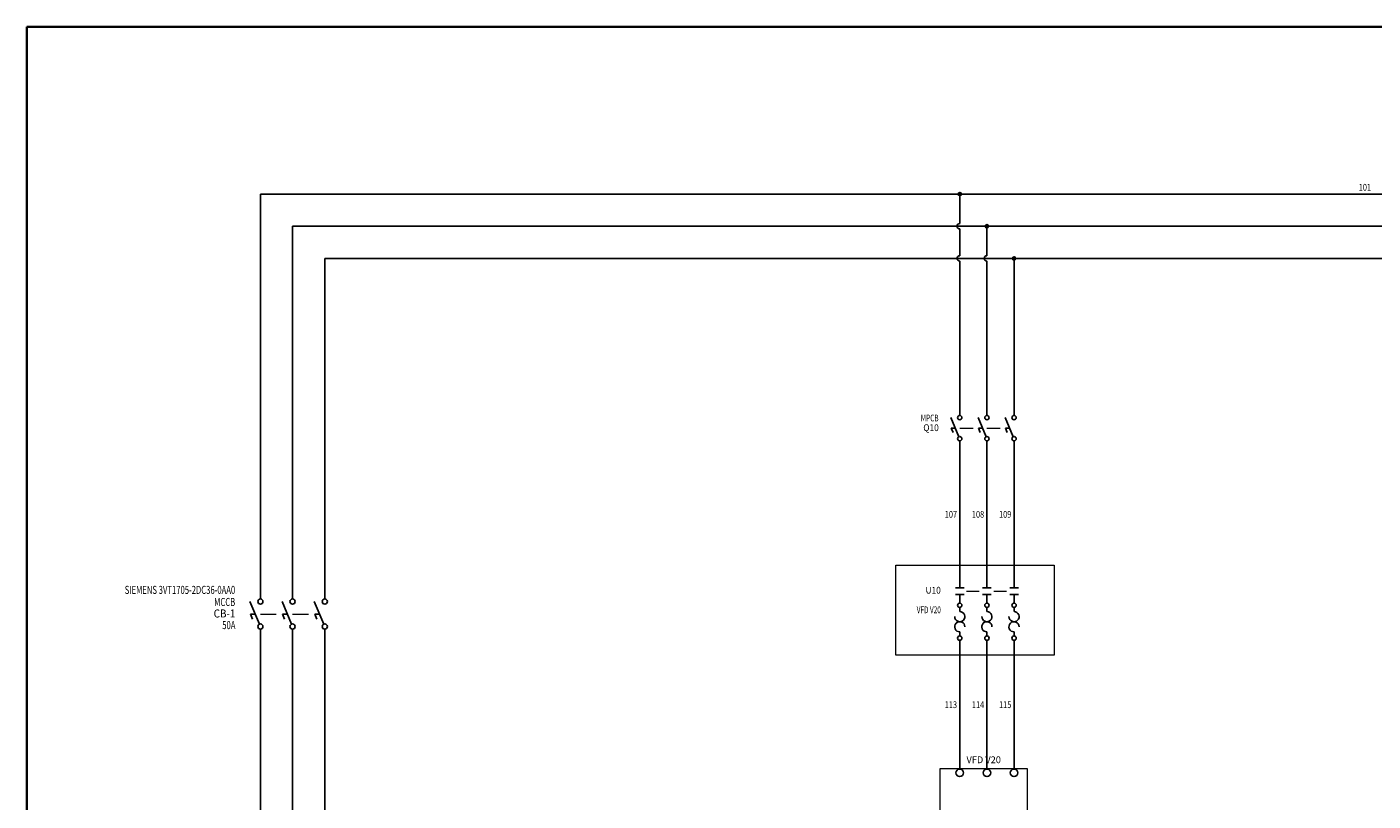
# Model space of a CAD drawing. Units: inches. Extents: x 12.5 to 62, y 4.7 to 37.4.
# Tile 3 of 5: x 12.5 to 37.3, y 23.1 to 37.4. Entities that reach past the tile are written whole.
import ezdxf
from ezdxf.enums import TextEntityAlignment as Align

# ---------------------------------------------------------------- set-up
doc = ezdxf.new("R2010")
doc.units = ezdxf.units.IN
doc.header["$MEASUREMENT"] = 0
for name, color, linetype, lineweight in [('16AWG-BLU', 182, 'Continuous', 25), ('16AWG-GRNYEL', 60, 'Continuous', 25), ('16AWG-RED', 1, 'Continuous', 25), ('E-ANNO-TEXT', 92, 'Continuous', 18), ('E-ANNO-TTLB', 7, 'Continuous', 35), ('LINK', 9, 'Continuous', 13), ('LOCBOX', 7, 'Continuous', 18), ('SYMS', 7, 'Continuous', 25), ('WIRENO', 72, 'Continuous', 18)]:
    doc.layers.add(name, color=color, linetype=linetype, lineweight=lineweight)
for name, color, linetype in [('DESCCHILD', 20, 'Continuous'), ('LOC', 8, 'Continuous'), ('MISC', 7, 'Continuous'), ('TAGS', 150, 'Continuous')]:
    doc.layers.add(name, color=color, linetype=linetype)
doc.styles.get("Standard").update_dxf_attribs({"font": 'arial.ttf'})
doc.styles.add('WD', font='romans.shx')

# ---------------------------------------------------------------- blocks, each defined once
blk = doc.blocks.new('VDS11')
for p, q in [((-0.016, -0.157), (-0.163, 0.195)), ((-0.081, 0), (-0.156, 0)), ((-0.124, -0.078), (-0.156, 0))]:
    blk.add_line(p, q)
for centre in [(0, 0.194), (0, -0.194)]:
    blk.add_circle(centre, 0.0403)
at = {"style": 'WD'}
for tag, width, p in [('INST', 0.7, (-0.391, 0.312)), ('LOC', 0.7, (-0.391, 0.125)), ('TAG1', 0.9, (-0.388, -0.054)), ('RATING1', 0.7, (-0.388, -0.234)), ('DESC1', 0.7, (-0.387, -0.422)), ('DESC2', 0.7, (-0.388, -0.609))]:
    blk.add_attdef(tag, text='', height=0.125, dxfattribs=dict(at, width=width)).set_placement(p, align=Align.RIGHT)
for tag, height, flags, p in [('TERM01', 0.125, 8, (-0.069, 0.258)), ('CONTACT', 0.0125, 9, (-0.083, -0.067)), ('FAMILY', 0.0125, 9, (-0.1, -0.046)), ('MFG', 0.0125, 9, (-0.1, -0.11)), ('CAT', 0.0125, 9, (-0.1, -0.091))]:
    blk.add_attdef(tag, text='', height=height, dxfattribs=dict(at, flags=flags)).set_placement(p, align=Align.RIGHT)
at = {"style": 'WD', "flags": 1}
for tag, p in [('X2TERM01', (0, 0.234)), ('X8TERM02', (0, -0.234))]:
    blk.add_attdef(tag, p, '', height=0.0125, dxfattribs=at)
at = {"style": 'WD'}
for tag, p in [('X4LINK', (-0.254, 0)), ('X1LINK', (0, 0))]:
    blk.add_attdef(tag, p, '', height=0.0125, dxfattribs=at)
at = {"style": 'WD', "width": 0.7}
blk.add_attdef('XREF', (0.161, -0.047), '', height=0.125, dxfattribs=at)
at = {"style": 'WD', "flags": 9}
blk.add_attdef('ASSYCODE', text='', height=0.0125, dxfattribs=at).set_placement((-0.115, -0.137), align=Align.CENTER)
at = {"style": 'WD', "flags": 8}
blk.add_attdef('TERM02', text='', height=0.125, dxfattribs=at).set_placement((-0.051, -0.267), align=Align.TOP_RIGHT)
blk = doc.blocks.new('VDS21')
for p, q in [((-0.016, -0.157), (-0.163, 0.195)), ((-0.081, 0), (-0.156, 0)), ((-0.124, -0.078), (-0.156, 0))]:
    blk.add_line(p, q)
for centre in [(0, 0.194), (0, -0.194)]:
    blk.add_circle(centre, 0.0403)
at = {"style": 'WD'}
for tag, width, p in [('INST', 0.7, (-0.373, 0.406)), ('LOC', 0.7, (-0.373, 0.221)), ('TAG2', 0.9, (-0.373, 0.031)), ('XREF', 0.7, (-0.37, -0.155)), ('DESC1', 0.7, (-0.37, -0.344)), ('DESC2', 0.7, (-0.37, -0.531))]:
    blk.add_attdef(tag, text='', height=0.125, dxfattribs=dict(at, width=width)).set_placement(p, align=Align.RIGHT)
for tag, height, flags, p in [('TERM01', 0.125, 8, (-0.069, 0.258)), ('CONTACT', 0.0125, 9, (-0.083, -0.106)), ('FAMILY', 0.0125, 9, (-0.1, -0.046))]:
    blk.add_attdef(tag, text='', height=height, dxfattribs=dict(at, flags=flags)).set_placement(p, align=Align.RIGHT)
at = {"style": 'WD', "flags": 1}
for tag, p in [('X2TERM01', (0, 0.234)), ('X8TERM02', (0, -0.234))]:
    blk.add_attdef(tag, p, '', height=0.0125, dxfattribs=at)
at = {"style": 'WD'}
for tag, p in [('X4LINK', (-0.254, 0)), ('X1LINK', (0, 0))]:
    blk.add_attdef(tag, p, '', height=0.0125, dxfattribs=at)
at = {"style": 'WD', "flags": 8}
blk.add_attdef('TERM02', text='', height=0.125, dxfattribs=at).set_placement((-0.051, -0.267), align=Align.TOP_RIGHT)
blk = doc.blocks.new('WDDOT')
for radius in [0.03, 0.0187, 0.00929]:
    blk.add_circle((0, 0), radius)
blk = doc.blocks.new('VMS21OL')
for p, q in [((-0.08, 0.062), (0.08, 0.062)), ((-0.08, -0.062), (0.08, -0.062)), ((0, -0.219), (0, -0.062)), ((0, -0.299), (0, -0.375)), ((0, -0.75), (0, -0.826))]:
    blk.add_line(p, q)
for centre in [(0, -0.259), (0, -0.866)]:
    blk.add_circle(centre, 0.04)
for centre, start, end in [((0, -0.469), 180.001, 90.002), ((0, -0.656), 0, 270.001)]:
    blk.add_arc(centre, 0.0938, start, end)
at = {"style": 'WD'}
for tag, width, p in [('INST', 0.7, (-0.352, 0.312)), ('LOC', 0.7, (-0.352, 0.125)), ('TAG2', 0.9, (-0.35, -0.045)), ('XREF', 0.7, (-0.348, -0.219)), ('DESC1', 0.7, (-0.348, -0.406)), ('DESC2', 0.7, (-0.348, -0.594)), ('DESC3', 0.7, (-0.348, -0.781))]:
    blk.add_attdef(tag, text='', height=0.125, dxfattribs=dict(at, width=width)).set_placement(p, align=Align.RIGHT)
at = {"style": 'WD', "width": 0.9, "flags": 8}
blk.add_attdef('TERM01', text='', height=0.125, dxfattribs=at).set_placement((-0.031, 0.125), align=Align.RIGHT)
at = {"style": 'WD'}
for tag, p, height, flags in [('FAMILY', (-0.181, 0.003), 0.01, 9), ('X2TERM01', (0, 0.062), 0.0125, 1), ('CONTACT', (-0.181, -0.014), 0.01, 1), ('X8TERM02', (0, -0.906), 0.0125, 1)]:
    blk.add_attdef(tag, p, '', height=height, dxfattribs=dict(at, flags=flags))
for tag, p in [('X4LINK', (-0.141, 0)), ('X1LINK', (0.125, 0))]:
    blk.add_attdef(tag, p, '', height=0.01, dxfattribs=at)
at = {"style": 'WD', "width": 0.9, "flags": 8}
blk.add_attdef('TERM02', text='', height=0.125, dxfattribs=at).set_placement((-0.031, -0.969), align=Align.TOP_RIGHT)
blk = doc.blocks.new('VT0_02')
blk.add_circle((0, 0), 0.0699)
at = {"style": 'WD', "flags": 1}
for tag, p in [('X4TERM01', (-0.07, 0)), ('X2TERM01', (0, 0.07)), ('X1TERM01', (0.07, 0)), ('X8TERM01', (0, -0.07))]:
    blk.add_attdef(tag, p, '', height=0.01, dxfattribs=at)
blk = doc.blocks.new('WD_WNH')
at = {"style": 'WD', "width": 0.8}
blk.add_attdef('WIRENO', text='', height=0.125, dxfattribs=at).set_placement((0, 0.062), align=Align.CENTER)
at = {"style": 'WD', "flags": 1}
for tag, p in [('W01USER', (0, 0.078)), ('W02USER', (0, 0.07)), ('W03USER', (0, 0.062)), ('W04USER', (0, 0.055)), ('W05USER', (0, 0.047)), ('W06USER', (0, 0.039)), ('W07USER', (0, 0.031)), ('W08USER', (0, 0.023)), ('W09USER', (0, 0.016)), ('W10USER', (0, 0.008))]:
    blk.add_attdef(tag, text='', height=0.005, dxfattribs=at).set_placement(p, align=Align.CENTER)
blk = doc.blocks.new('WD_WNV')
at = {"style": 'WD', "width": 0.8}
blk.add_attdef('WIRENO', text='', height=0.125, dxfattribs=at).set_placement((-0.05, 0), align=Align.MIDDLE_RIGHT)
at = {"style": 'WD', "flags": 1}
for tag, p in [('W01USER', (-0.062, 0.094)), ('W02USER', (-0.062, 0.086)), ('W03USER', (-0.062, 0.078)), ('W04USER', (-0.062, 0.07)), ('W05USER', (-0.062, 0.062)), ('W06USER', (-0.062, 0.055)), ('W07USER', (-0.062, 0.047)), ('W08USER', (-0.062, 0.039)), ('W09USER', (-0.062, 0.031)), ('W10USER', (-0.062, 0.023))]:
    blk.add_attdef(tag, text='', height=0.005, dxfattribs=at).set_placement(p, align=Align.CENTER)

msp = doc.modelspace()

# ---------------------------------------------------------------- linework, layer by layer
at = {"layer": '16AWG-BLU'}
for p, q in [((57.548, 33.109), (18.014, 33.109)), ((18.014, 33.109), (18.014, 26.83)), ((30.719, 33.109), (30.719, 30.214)), ((30.719, 29.745), (30.719, 27.035)), ((18.014, 26.274), (18.014, 17.161)), ((30.719, 26.067), (30.719, 23.694))]:
    msp.add_line(p, q, dxfattribs=at)
at = {"layer": '16AWG-GRNYEL'}
for p, q in [((57.548, 33.703), (17.421, 33.703)), ((17.421, 33.703), (17.421, 26.83)), ((30.219, 33.703), (30.219, 33.159)), ((30.219, 33.059), (30.219, 30.214)), ((30.219, 29.745), (30.219, 27.035)), ((17.421, 26.274), (17.421, 17.161)), ((30.219, 26.067), (30.219, 23.694))]:
    msp.add_line(p, q, dxfattribs=at)
msp.add_arc((30.219, 33.109), 0.05, 90, 270, dxfattribs=at)
at = {"layer": '16AWG-RED'}
for p, q in [((57.544, 34.296), (16.828, 34.296)), ((16.828, 34.296), (16.828, 26.83)), ((29.719, 34.296), (29.719, 33.753)), ((29.719, 33.653), (29.719, 33.159)), ((29.719, 33.059), (29.719, 30.214)), ((29.719, 29.745), (29.719, 27.035)), ((16.828, 26.274), (16.828, 17.161)), ((29.719, 26.067), (29.719, 23.694))]:
    msp.add_line(p, q, dxfattribs=at)
for centre in [(29.719, 33.703), (29.719, 33.109)]:
    msp.add_arc(centre, 0.05, 90, 270, dxfattribs=at)
at = {"layer": 'E-ANNO-TTLB'}
msp.add_lwpolyline([(12.524, 37.377), (62.033, 37.377), (62.033, 4.741), (12.524, 4.741)], close=True, dxfattribs=at)
at = {"layer": 'LINK'}
for points in [[(29.719, 29.979), (29.965, 29.979)], [(30.219, 29.979), (30.465, 29.979)], [(29.844, 26.973), (30.078, 26.973)], [(30.344, 26.973), (30.578, 26.973)], [(16.828, 26.552), (17.12, 26.552)], [(17.421, 26.552), (17.713, 26.552)]]:
    msp.add_lwpolyline(points, dxfattribs=at)
at = {"layer": 'LOCBOX'}
for points in [[(28.542, 27.454), (31.461, 27.454), (31.461, 25.791), (28.542, 25.791)], [(29.357, 23.701), (30.964, 23.701), (30.964, 22.632), (29.357, 22.632)]]:
    msp.add_lwpolyline(points, close=True, dxfattribs=at)

# ---------------------------------------------------------------- block references
at = {"layer": 'SYMS'}
for name, p in [('WDDOT', (29.719, 34.296)), ('WDDOT', (30.219, 33.703)), ('WDDOT', (30.719, 33.109)), ('VDS21', (30.219, 29.979)), ('VDS21', (30.719, 29.979)), ('VMS21OL', (30.219, 26.973)), ('VMS21OL', (30.719, 26.973)), ('VT0_02', (29.719, 23.624)), ('VT0_02', (30.22, 23.624)), ('VT0_02', (30.719, 23.624))]:
    msp.add_blockref(name, p, dxfattribs=at)
ref = msp.add_blockref('VDS11', (29.719, 29.979), dxfattribs=at)
ref.add_attrib('TAG1', 'Q10', dxfattribs={"layer": 'TAGS', "height": 0.125, "style": 'WD', "width": 0.9}).set_placement((29.331, 29.925), align=Align.RIGHT)
ref.add_attrib('LOC', 'MPCB', dxfattribs={"layer": 'LOC', "height": 0.125, "style": 'WD', "width": 0.7}).set_placement((29.328, 30.104), align=Align.RIGHT)
ref = msp.add_blockref('VDS11', (16.828, 26.552), dxfattribs=dict(at, xscale=1.186465831832244, yscale=1.186465831832244, zscale=1.186465831832244))
ref.add_attrib('INST', 'SIEMENS 3VT1705-2DC36-0AA0', dxfattribs={"layer": 'LOC', "height": 0.14831, "style": 'WD', "width": 0.7}).set_placement((16.364, 26.923), align=Align.RIGHT)
ref.add_attrib('TAG1', 'CB-1', dxfattribs={"layer": 'TAGS', "height": 0.1483, "style": 'WD', "width": 0.9}).set_placement((16.367, 26.488), align=Align.RIGHT)
ref.add_attrib('LOC', 'MCCB', dxfattribs={"layer": 'LOC', "height": 0.1483, "style": 'WD', "width": 0.7}).set_placement((16.364, 26.7), align=Align.RIGHT)
ref.add_attrib('RATING1', '50A', dxfattribs={"layer": 'MISC', "height": 0.1483, "style": 'WD', "width": 0.7}).set_placement((16.368, 26.274), align=Align.RIGHT)
ref = msp.add_blockref('VMS21OL', (29.719, 26.973), dxfattribs=at)
ref.add_attrib('DESC1', 'VFD V20', dxfattribs={"layer": 'DESCCHILD', "height": 0.125, "style": 'WD', "width": 0.7}).set_placement((29.37, 26.567), align=Align.RIGHT)
ref.add_attrib('TAG2', 'U10', dxfattribs={"layer": 'TAGS', "height": 0.125, "style": 'WD', "width": 0.9}).set_placement((29.369, 26.928), align=Align.RIGHT)
at = {"layer": 'SYMS', "xscale": 1.186465831832244, "yscale": 1.186465831832244, "zscale": 1.186465831832244}
for p in [(17.421, 26.552), (18.014, 26.552)]:
    msp.add_blockref('VDS21', p, dxfattribs=at)
at = {"layer": 'WIRENO'}
ref = msp.add_blockref('WD_WNH', (37.186, 34.296), dxfattribs=at)
ref.add_attrib('WIRENO', '101', dxfattribs={"linetype": 'Continuous', "height": 0.125, "style": 'WD', "width": 0.8}).set_placement((37.186, 34.358), align=Align.CENTER)
ref = msp.add_blockref('WD_WNV', (29.719, 28.39), dxfattribs=at)
ref.add_attrib('WIRENO', '107', dxfattribs={"linetype": 'Continuous', "height": 0.125, "style": 'WD', "width": 0.8}).set_placement((29.669, 28.39), align=Align.MIDDLE_RIGHT)
ref = msp.add_blockref('WD_WNV', (30.219, 28.39), dxfattribs=at)
ref.add_attrib('WIRENO', '108', dxfattribs={"linetype": 'Continuous', "height": 0.125, "style": 'WD', "width": 0.8}).set_placement((30.169, 28.39), align=Align.MIDDLE_RIGHT)
ref = msp.add_blockref('WD_WNV', (30.719, 28.39), dxfattribs=at)
ref.add_attrib('WIRENO', '109', dxfattribs={"linetype": 'Continuous', "height": 0.125, "style": 'WD', "width": 0.8}).set_placement((30.669, 28.39), align=Align.MIDDLE_RIGHT)
ref = msp.add_blockref('WD_WNV', (29.719, 24.88), dxfattribs=at)
ref.add_attrib('WIRENO', '113', dxfattribs={"linetype": 'Continuous', "height": 0.125, "style": 'WD', "width": 0.8}).set_placement((29.669, 24.88), align=Align.MIDDLE_RIGHT)
ref = msp.add_blockref('WD_WNV', (30.219, 24.88), dxfattribs=at)
ref.add_attrib('WIRENO', '114', dxfattribs={"linetype": 'Continuous', "height": 0.125, "style": 'WD', "width": 0.8}).set_placement((30.169, 24.88), align=Align.MIDDLE_RIGHT)
ref = msp.add_blockref('WD_WNV', (30.719, 24.88), dxfattribs=at)
ref.add_attrib('WIRENO', '115', dxfattribs={"linetype": 'Continuous', "height": 0.125, "style": 'WD', "width": 0.8}).set_placement((30.669, 24.88), align=Align.MIDDLE_RIGHT)

# ---------------------------------------------------------------- texts
at = {"layer": 'E-ANNO-TEXT'}
msp.add_text('VFD V20', height=0.125, dxfattribs=at).set_placement((30.16, 23.763), align=Align.BOTTOM_CENTER)

doc.saveas('drawing.dxf')
